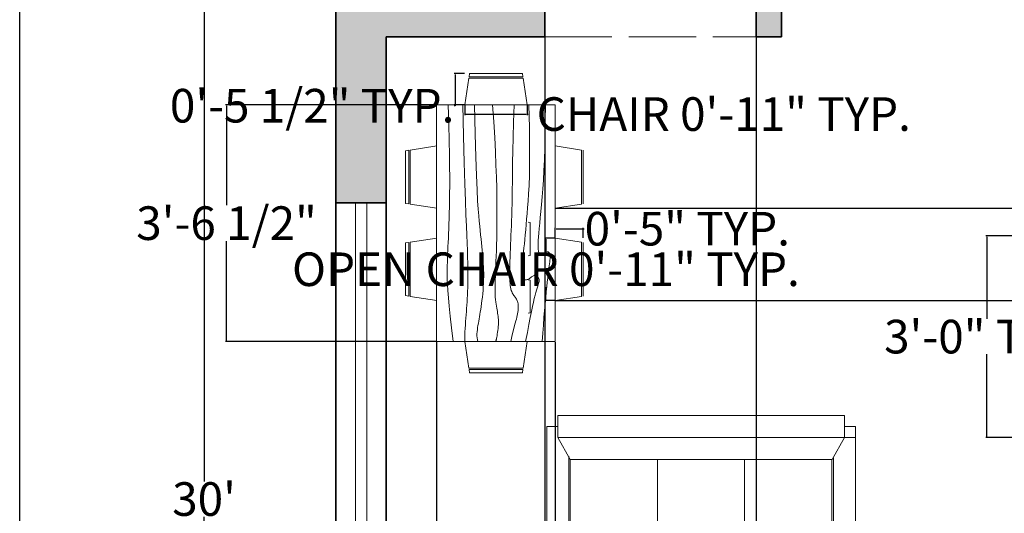
# Model space of a CAD drawing. Units: inches. Extents: x 335 to 688, y 1043 to 1486.
# Tile 3 of 7: x 335 to 510, y 1258 to 1347. Entities that reach past the tile are written whole.
import ezdxf

# ---------------------------------------------------------------- set-up
doc = ezdxf.new("R2010")
doc.units = ezdxf.units.IN
doc.header["$MEASUREMENT"] = 0
doc.linetypes.add('ACAD_ISO02W100', pattern=[15, 12, -3])
for name, color, linetype, lineweight in [('A-ANNO-DIMS', 2, 'Continuous', 18), ('A-ANNO-TTLB', 7, 'Continuous', 25), ('A-FURN', 8, 'Continuous', 18), ('A-GLAZ', 4, 'Continuous', 18), ('A-WALL', 7, 'Continuous', 35), ('A-WALL-OVHD', 7, 'ACAD_ISO02W100', 18), ('A-WALL-PATT', 252, 'Continuous', 13)]:
    doc.layers.add(name, color=color, linetype=linetype, lineweight=lineweight)
doc.styles.get("Standard").update_dxf_attribs({"font": 'arial.ttf'})
doc.dimstyles.get("Standard").update_dxf_attribs({"dimtxt": 6, "dimasz": 0.18, "dimexe": 0.18, "dimexo": 0.0625, "dimgap": 0.09, "dimtad": 0, "dimtih": 1, "dimtoh": 1, "dimdec": 1, "dimzin": 0, "dimdsep": 46, "dimlunit": 3, "dimtxsty": 'Standard', "dimcen": 0.09, "dimadec": 0, "dimazin": 0, "dimtfac": 1, "dimtdec": 1, "dimtofl": 0, "dimtmove": 0, "dimatfit": 3, "dimfxl": 1, "dimtolj": 1, "dimtzin": 0, "dimarcsym": 0})

# ---------------------------------------------------------------- blocks, each defined once
blk = doc.blocks.new('*D4')
at = {"layer": 'A-ANNO-DIMS', "color": 0, "lineweight": -2, "transparency": 16777216}
for p, q in [((391.04, 1440.97), (367.42, 1440.97)), ((367.6, 1440.79), (367.6, 1264.12)), ((367.6, 1081.15), (367.6, 1257.81)), ((391.04, 1080.97), (367.42, 1080.97))]:
    blk.add_line(p, q, dxfattribs=at)
at = {"layer": 'A-ANNO-DIMS', "color": 0, "transparency": 16777216}
for points in [[(367.57, 1440.79), (367.63, 1440.79), (367.6, 1440.97)], [(367.57, 1081.15), (367.63, 1081.15), (367.6, 1080.97)]]:
    blk.add_solid(points, dxfattribs=at)
at = {"layer": 'Defpoints', "color": 0, "transparency": 16777216}
for p in [(391.11, 1440.97), (367.6, 1080.97), (391.11, 1080.97)]:
    blk.add_point(p, dxfattribs=at)
at = {"layer": 'A-ANNO-DIMS', "color": 0, "transparency": 16777216, "insert": (367.6, 1260.97), "char_height": 6, "attachment_point": 5}
blk.add_mtext("\\A1;30'", dxfattribs=at)
blk = doc.blocks.new('SOFA-THREE-SEAT')
for p, q in [((53.08, 22.23), (1.96, 22.23)), ((1.96, 18.31), (1.96, 22.23)), ((53.08, 18.31), (53.08, 22.23)), ((0, 20.27), (0, 0)), ((1.96, 20.27), (0, 20.27)), ((55.04, 20.27), (53.08, 20.27)), ((55.04, 20.27), (55.04, 0)), ((55.04, 18.31), (1.96, 18.31)), ((4.17, 14.38), (1.96, 18.31)), ((53.08, 18.31), (50.88, 14.38)), ((3.92, 14.94), (3.92, 0)), ((19.74, 0.65), (19.74, 14.38)), ((35.3, 0.65), (35.3, 14.38)), ((50.87, 0.65), (50.87, 14.38)), ((51.12, 14.69), (51.12, 0)), ((3.92, 0), (0, 0)), ((51.12, 0), (55.04, 0))]:
    blk.add_line(p, q)
blk.add_lwpolyline([(50.88, 14.38), (4.17, 14.38), (4.17, 0.65), (50.87, 0.65)])
blk = doc.blocks.new('CHAIR-DINING')
for p, q in [((0.88, 10.41), (5.59, 11.15)), ((0, 10.28), (0.59, 10.37)), ((0, 10.28), (0, 0.87)), ((0.59, 0.78), (0.59, 10.37)), ((0.88, 10.41), (0.88, 0.73)), ((0.59, 0.78), (0, 0.87)), ((5.59, 0), (0.88, 0.73))]:
    blk.add_line(p, q)
blk = doc.blocks.new('CHAIR-DINING-OPEN')
for p, q in [((4.7, 10.41), (0, 11.15)), ((4.7, 10.41), (4.7, 0.73)), ((5, 0.78), (5, 10.37)), ((0, 0), (4.7, 0.73))]:
    blk.add_line(p, q)
blk = doc.blocks.new('WIN-60IN')
for p, q in [((0, 0), (0, 60)), ((3.5, 0), (3.5, 60)), ((5.5, 60), (5.5, 0)), ((9, 60), (9, 0))]:
    blk.add_line(p, q)
blk = doc.blocks.new('*D21')
at = {"layer": 'A-ANNO-DIMS', "color": 0, "lineweight": -2, "transparency": 16777216}
for p, q in [((414.1, 1331.32), (414.1, 1329.53)), ((425.25, 1331.32), (425.25, 1329.53)), ((414.28, 1329.71), (425.07, 1329.71)), ((425.25, 1329.71), (425.43, 1329.71))]:
    blk.add_line(p, q, dxfattribs=at)
at = {"layer": 'A-ANNO-DIMS', "color": 0, "transparency": 16777216}
for points in [[(414.28, 1329.74), (414.28, 1329.68), (414.1, 1329.71)], [(425.07, 1329.74), (425.07, 1329.68), (425.25, 1329.71)]]:
    blk.add_solid(points, dxfattribs=at)
at = {"layer": 'Defpoints', "color": 0, "transparency": 16777216}
for p in [(414.1, 1331.38), (425.25, 1331.38), (425.25, 1329.71)]:
    blk.add_point(p, dxfattribs=at)
at = {"layer": 'A-ANNO-DIMS', "color": 0, "transparency": 16777216, "insert": (460.3, 1329.71), "char_height": 6, "attachment_point": 5}
blk.add_mtext('\\A1;CHAIR 0\'-11" TYP.', dxfattribs=at)
blk = doc.blocks.new('*D22')
at = {"layer": 'A-ANNO-DIMS', "color": 0, "lineweight": -2, "transparency": 16777216}
for p, q in [((414.03, 1336.97), (412.24, 1336.97)), ((412.42, 1336.79), (412.42, 1331.56)), ((414.03, 1331.38), (412.24, 1331.38)), ((412.42, 1331.38), (412.42, 1331.2)), ((412.42, 1331.2), (412.24, 1331.2))]:
    blk.add_line(p, q, dxfattribs=at)
at = {"layer": 'A-ANNO-DIMS', "color": 0, "transparency": 16777216}
for points in [[(412.39, 1336.79), (412.45, 1336.79), (412.42, 1336.97)], [(412.39, 1331.56), (412.45, 1331.56), (412.42, 1331.38)]]:
    blk.add_solid(points, dxfattribs=at)
at = {"layer": 'Defpoints', "color": 0, "transparency": 16777216}
for p in [(414.1, 1336.97), (412.42, 1331.38), (414.1, 1331.38)]:
    blk.add_point(p, dxfattribs=at)
at = {"layer": 'A-ANNO-DIMS', "color": 0, "transparency": 16777216, "insert": (386.88, 1331.2), "char_height": 6, "attachment_point": 5}
blk.add_mtext('\\A1;0\'-5 1/2" TYP.', dxfattribs=at)
blk = doc.blocks.new('*D23')
at = {"layer": 'A-ANNO-DIMS', "color": 0, "lineweight": -2, "transparency": 16777216}
for p, q in [((430.19, 1307.57), (428.4, 1307.57)), ((428.58, 1307.39), (428.58, 1305.19)), ((428.58, 1296.6), (428.58, 1298.8)), ((430.19, 1296.42), (428.4, 1296.42))]:
    blk.add_line(p, q, dxfattribs=at)
at = {"layer": 'A-ANNO-DIMS', "color": 0, "transparency": 16777216}
for points in [[(428.55, 1307.39), (428.61, 1307.39), (428.58, 1307.57)], [(428.55, 1296.6), (428.61, 1296.6), (428.58, 1296.42)]]:
    blk.add_solid(points, dxfattribs=at)
at = {"layer": 'Defpoints', "color": 0, "transparency": 16777216}
for p in [(428.58, 1307.57), (430.25, 1307.57), (430.25, 1296.42)]:
    blk.add_point(p, dxfattribs=at)
at = {"layer": 'A-ANNO-DIMS', "color": 0, "transparency": 16777216, "insert": (428.58, 1302), "char_height": 6, "attachment_point": 5}
blk.add_mtext('\\A1;OPEN CHAIR 0\'-11" TYP.', dxfattribs=at)
blk = doc.blocks.new('*D24')
at = {"layer": 'A-ANNO-DIMS', "color": 0, "lineweight": -2, "transparency": 16777216}
for p, q in [((430.25, 1307.63), (430.25, 1309.42)), ((430.43, 1309.24), (435.07, 1309.24)), ((435.25, 1307.63), (435.25, 1309.42)), ((435.25, 1309.24), (435.43, 1309.24))]:
    blk.add_line(p, q, dxfattribs=at)
at = {"layer": 'A-ANNO-DIMS', "color": 0, "transparency": 16777216}
for points in [[(430.43, 1309.27), (430.43, 1309.21), (430.25, 1309.24)], [(435.07, 1309.27), (435.07, 1309.21), (435.25, 1309.24)]]:
    blk.add_solid(points, dxfattribs=at)
at = {"layer": 'Defpoints', "color": 0, "transparency": 16777216}
for p in [(435.25, 1309.24), (430.25, 1307.57), (435.25, 1307.57)]:
    blk.add_point(p, dxfattribs=at)
at = {"layer": 'A-ANNO-DIMS', "color": 0, "transparency": 16777216, "insert": (453.8, 1309.24), "char_height": 6, "attachment_point": 5}
blk.add_mtext('\\A1;0\'-5" TYP.', dxfattribs=at)
blk = doc.blocks.new('*D32')
at = {"layer": 'A-ANNO-DIMS', "color": 0, "lineweight": -2, "transparency": 16777216}
for p, q in [((512.54, 1307.97), (507.03, 1307.97)), ((507.21, 1307.79), (507.21, 1293.12)), ((507.21, 1272.15), (507.21, 1286.81)), ((512.54, 1271.97), (507.03, 1271.97))]:
    blk.add_line(p, q, dxfattribs=at)
at = {"layer": 'A-ANNO-DIMS', "color": 0, "transparency": 16777216}
for points in [[(507.18, 1307.79), (507.24, 1307.79), (507.21, 1307.97)], [(507.18, 1272.15), (507.24, 1272.15), (507.21, 1271.97)]]:
    blk.add_solid(points, dxfattribs=at)
at = {"layer": 'Defpoints', "color": 0, "transparency": 16777216}
for p in [(507.21, 1307.97), (512.61, 1307.97), (512.61, 1271.97)]:
    blk.add_point(p, dxfattribs=at)
at = {"layer": 'A-ANNO-DIMS', "color": 0, "transparency": 16777216, "insert": (507.21, 1289.97), "char_height": 6, "attachment_point": 5}
blk.add_mtext('\\A1;3\'-0" TYP.', dxfattribs=at)
blk = doc.blocks.new('*D39')
at = {"layer": 'A-ANNO-DIMS', "color": 0, "lineweight": -2, "transparency": 16777216}
for p, q in [((409.09, 1289), (409.09, 1061.29)), ((430.25, 1289), (430.25, 1061.29)), ((409.27, 1061.47), (411.89, 1061.47)), ((430.07, 1061.47), (427.45, 1061.47))]:
    blk.add_line(p, q, dxfattribs=at)
at = {"layer": 'A-ANNO-DIMS', "color": 0, "transparency": 16777216}
for points in [[(409.27, 1061.5), (409.27, 1061.44), (409.09, 1061.47)], [(430.07, 1061.5), (430.07, 1061.44), (430.25, 1061.47)]]:
    blk.add_solid(points, dxfattribs=at)
at = {"layer": 'Defpoints', "color": 0, "transparency": 16777216}
for p in [(409.09, 1289.07), (430.25, 1289.07), (430.25, 1061.47)]:
    blk.add_point(p, dxfattribs=at)
at = {"layer": 'A-ANNO-DIMS', "color": 0, "transparency": 16777216, "insert": (419.67, 1061.47), "char_height": 6, "attachment_point": 5}
blk.add_mtext('\\A1;1\'-9"', dxfattribs=at)
blk = doc.blocks.new('*D40')
at = {"layer": 'A-ANNO-DIMS', "color": 0, "lineweight": -2, "transparency": 16777216}
for p, q in [((409.03, 1331.38), (371.43, 1331.38)), ((371.61, 1331.2), (371.61, 1313.42)), ((371.61, 1289.25), (371.61, 1307.03)), ((409.03, 1289.07), (371.43, 1289.07))]:
    blk.add_line(p, q, dxfattribs=at)
at = {"layer": 'A-ANNO-DIMS', "color": 0, "transparency": 16777216}
for points in [[(371.58, 1331.2), (371.64, 1331.2), (371.61, 1331.38)], [(371.58, 1289.25), (371.64, 1289.25), (371.61, 1289.07)]]:
    blk.add_solid(points, dxfattribs=at)
at = {"layer": 'Defpoints', "color": 0, "transparency": 16777216}
for p in [(371.61, 1331.38), (409.09, 1331.38), (409.09, 1289.07)]:
    blk.add_point(p, dxfattribs=at)
at = {"layer": 'A-ANNO-DIMS', "color": 0, "transparency": 16777216, "insert": (371.61, 1310.23), "char_height": 6, "attachment_point": 5}
blk.add_mtext('\\A1;3\'-6 1/2"', dxfattribs=at)
blk = doc.blocks.new('*D41')
at = {"layer": 'A-ANNO-DIMS', "color": 0, "lineweight": -2, "transparency": 16777216}
for p, q in [((430.31, 1312.88), (650.79, 1312.88)), ((650.61, 1312.7), (650.61, 1307.84)), ((650.61, 1296.6), (650.61, 1301.46)), ((430.31, 1296.42), (650.79, 1296.42))]:
    blk.add_line(p, q, dxfattribs=at)
at = {"layer": 'A-ANNO-DIMS', "color": 0, "transparency": 16777216}
for points in [[(650.58, 1312.7), (650.64, 1312.7), (650.61, 1312.88)], [(650.58, 1296.6), (650.64, 1296.6), (650.61, 1296.42)]]:
    blk.add_solid(points, dxfattribs=at)
at = {"layer": 'Defpoints', "color": 0, "transparency": 16777216}
for p in [(430.25, 1312.88), (650.61, 1312.88), (430.25, 1296.42)]:
    blk.add_point(p, dxfattribs=at)
at = {"layer": 'A-ANNO-DIMS', "color": 0, "transparency": 16777216, "insert": (650.61, 1304.65), "char_height": 6, "attachment_point": 5}
blk.add_mtext('\\A1;1\'-4 1/2"', dxfattribs=at)
blk = doc.blocks.new('*D60')
at = {"layer": 'A-ANNO-DIMS', "color": 0, "lineweight": -2, "transparency": 16777216}
for p, q in [((400.11, 1343.4), (400.11, 1061.29)), ((428.36, 1343.4), (428.36, 1061.29)), ((400.29, 1061.47), (428.18, 1061.47)), ((428.36, 1061.47), (428.54, 1061.47))]:
    blk.add_line(p, q, dxfattribs=at)
at = {"layer": 'A-ANNO-DIMS', "color": 0, "transparency": 16777216}
for points in [[(400.29, 1061.5), (400.29, 1061.44), (400.11, 1061.47)], [(428.18, 1061.5), (428.18, 1061.44), (428.36, 1061.47)]]:
    blk.add_solid(points, dxfattribs=at)
at = {"layer": 'Defpoints', "color": 0, "transparency": 16777216}
for p in [(400.11, 1343.47), (428.36, 1343.47), (428.36, 1061.47)]:
    blk.add_point(p, dxfattribs=at)
at = {"layer": 'A-ANNO-DIMS', "color": 0, "transparency": 16777216, "insert": (443.65, 1061.47), "char_height": 6, "attachment_point": 5}
blk.add_mtext('\\A1;2\'-4 1/2"', dxfattribs=at)
blk = doc.blocks.new('*D61')
at = {"layer": 'A-ANNO-DIMS', "color": 0, "lineweight": -2, "transparency": 16777216}
for p, q in [((428.36, 1347.9), (428.36, 1061.29)), ((466.11, 1347.9), (466.11, 1061.29)), ((428.54, 1061.47), (432.18, 1061.47)), ((465.93, 1061.47), (462.29, 1061.47))]:
    blk.add_line(p, q, dxfattribs=at)
at = {"layer": 'A-ANNO-DIMS', "color": 0, "transparency": 16777216}
for points in [[(428.54, 1061.5), (428.54, 1061.44), (428.36, 1061.47)], [(465.93, 1061.5), (465.93, 1061.44), (466.11, 1061.47)]]:
    blk.add_solid(points, dxfattribs=at)
at = {"layer": 'Defpoints', "color": 0, "transparency": 16777216}
for p in [(428.36, 1347.97), (466.11, 1347.97), (466.11, 1061.47)]:
    blk.add_point(p, dxfattribs=at)
at = {"layer": 'A-ANNO-DIMS', "color": 0, "transparency": 16777216, "insert": (447.24, 1061.47), "char_height": 6, "attachment_point": 5}
blk.add_mtext('\\A1;3\'-1 1/2"', dxfattribs=at)

msp = doc.modelspace()

# ---------------------------------------------------------------- hatches: boundary and pattern name
at = {"layer": 'A-WALL-PATT'}
h = msp.add_hatch(color=256, dxfattribs=at)
h.dxf.hatch_style = 1
h.paths.add_polyline_path([(478.71, 1440.97), (391.11, 1440.97), (391.11, 1411.42), (400.11, 1411.42), (400.11, 1431.97), (466.11, 1431.97), (466.11, 1347.97), (466.11, 1343.47), (470.61, 1343.47), (470.61, 1367.47), (512.61, 1367.47), (512.61, 1350.97), (517.11, 1350.97), (517.11, 1372.97), (512.61, 1372.97), (512.61, 1371.97), (470.61, 1371.97), (470.61, 1431.97), (478.71, 1431.97)])
h.paths.add_polyline_path([(631.11, 1440.97), (502.71, 1440.97), (502.71, 1431.97), (512.61, 1431.97), (512.61, 1404.97), (517.11, 1404.97), (517.11, 1431.97), (622.11, 1431.97), (622.11, 1401.6), (631.11, 1401.6)])
h.paths.add_polyline_path([(631.11, 1341.6), (622.11, 1341.6), (622.11, 1313.47), (517.11, 1313.47), (517.11, 1314.47), (512.61, 1314.47), (512.61, 1313.47), (512.61, 1307.97), (517.11, 1307.97), (517.11, 1308.97), (553.11, 1308.97), (553.11, 1262.47), (558.61, 1262.47), (558.61, 1266.97), (557.61, 1266.97), (557.61, 1308.97), (622.11, 1308.97), (622.11, 1297.63), (631.11, 1297.63)])
h.paths.add_polyline_path([(631.11, 1273.63), (622.11, 1273.63), (622.11, 1266.97), (590.61, 1266.97), (590.61, 1262.47), (622.11, 1262.47), (622.11, 1230.86), (631.11, 1230.86)])
h.paths.add_polyline_path([(400.11, 1253.85), (391.11, 1253.85), (391.11, 1132.26), (400.11, 1132.26), (400.11, 1149.97), (411.11, 1149.97), (411.11, 1154.47), (400.11, 1154.47)], flags=17)
h.paths.add_polyline_path([(400.11, 1375.42), (391.11, 1375.42), (391.11, 1313.85), (400.11, 1313.85), (400.11, 1343.47), (428.36, 1343.47), (428.36, 1347.97), (400.11, 1347.97)])

# ---------------------------------------------------------------- linework, layer by layer
at = {"layer": 'A-ANNO-TTLB'}
msp.add_lwpolyline([(334.72, 1486.4), (681.01, 1486.4), (681.01, 1043.03), (334.72, 1043.03)], close=True, dxfattribs=at)
at = {"layer": 'A-FURN'}
for p, q in [((409.09, 1331.38), (409.09, 1289.07)), ((430.25, 1331.38), (409.09, 1331.38)), ((430.25, 1289.07), (430.25, 1331.38)), ((425.76, 1310.32), (425.4, 1310.38)), ((425.76, 1310.32), (425.76, 1304.46)), ((425.4, 1304.4), (425.76, 1304.46)), ((425.76, 1300.06), (425.4, 1300.12)), ((425.76, 1300.06), (425.76, 1294.2)), ((425.4, 1294.14), (425.76, 1294.2)), ((409.09, 1289.07), (430.25, 1289.07))]:
    msp.add_line(p, q, dxfattribs=at)
for points in [[(411.15, 1331.38), (411.25, 1327.91), (411.32, 1324.94), (411.37, 1322.41), (411.4, 1320.26), (411.42, 1318.44), (411.42, 1316.87), (411.41, 1315.5), (411.39, 1314.27), (411.37, 1313.12), (411.35, 1312.04), (411.32, 1311.03), (411.29, 1310.08), (411.26, 1309.19), (411.22, 1308.35), (411.19, 1307.55), (411.15, 1306.8), (411.11, 1306.08), (411.08, 1305.39), (411.05, 1304.71), (411.02, 1304.03), (411, 1303.34), (410.98, 1302.63), (410.97, 1301.88), (410.98, 1301.09), (410.99, 1300.24), (411.03, 1299.29), (411.09, 1298.19), (411.18, 1296.91), (411.32, 1295.4), (411.5, 1293.61), (411.73, 1291.52), (412.03, 1289.07)], [(413.79, 1331.38), (413.9, 1325.74), (414.01, 1321.08), (414.12, 1317.27), (414.22, 1314.19), (414.31, 1311.71), (414.39, 1309.71), (414.47, 1308.06), (414.53, 1306.65), (414.58, 1305.36), (414.61, 1304.17), (414.64, 1303.07), (414.65, 1302.06), (414.66, 1301.12), (414.65, 1300.26), (414.64, 1299.46), (414.63, 1298.72), (414.61, 1298.02), (414.58, 1297.37), (414.55, 1296.76), (414.52, 1296.16), (414.48, 1295.59), (414.44, 1295.02), (414.4, 1294.45), (414.36, 1293.87), (414.31, 1293.27), (414.26, 1292.66), (414.22, 1292.05), (414.18, 1291.43), (414.14, 1290.82), (414.11, 1290.22), (414.09, 1289.63), (414.09, 1289.07)], [(415.85, 1331.38), (415.96, 1326.2), (416.07, 1322.03), (416.18, 1318.73), (416.29, 1316.17), (416.39, 1314.21), (416.49, 1312.72), (416.59, 1311.56), (416.68, 1310.59), (416.77, 1309.71), (416.86, 1308.89), (416.94, 1308.12), (417.01, 1307.39), (417.09, 1306.7), (417.15, 1306.04), (417.21, 1305.4), (417.27, 1304.79), (417.32, 1304.19), (417.37, 1303.6), (417.41, 1303.02), (417.44, 1302.44), (417.47, 1301.86), (417.48, 1301.28), (417.48, 1300.69), (417.47, 1300.09), (417.44, 1299.48), (417.41, 1298.86), (417.36, 1298.24), (417.3, 1297.62), (417.24, 1297.02), (417.17, 1296.43), (417.1, 1295.87), (417.03, 1295.34), (416.95, 1294.84), (416.88, 1294.37), (416.81, 1293.94), (416.74, 1293.52), (416.66, 1293.12), (416.6, 1292.74), (416.53, 1292.36), (416.46, 1291.98), (416.4, 1291.6), (416.35, 1291.23), (416.3, 1290.85), (416.28, 1290.48), (416.27, 1290.11), (416.29, 1289.75), (416.35, 1289.4), (416.44, 1289.07)], [(419.08, 1331.38), (419.28, 1328.32), (419.45, 1325.52), (419.58, 1322.95), (419.67, 1320.6), (419.75, 1318.45), (419.8, 1316.49), (419.83, 1314.68), (419.84, 1313.02), (419.85, 1311.48), (419.84, 1310.06), (419.82, 1308.74), (419.8, 1307.51), (419.77, 1306.37), (419.74, 1305.31), (419.71, 1304.31), (419.67, 1303.37), (419.63, 1302.47), (419.6, 1301.62), (419.57, 1300.82), (419.54, 1300.07), (419.52, 1299.36), (419.51, 1298.71), (419.51, 1298.1), (419.52, 1297.54), (419.55, 1297.03), (419.59, 1296.57), (419.63, 1296.15), (419.68, 1295.76), (419.74, 1295.4), (419.8, 1295.07), (419.86, 1294.75), (419.92, 1294.45), (419.97, 1294.17), (420.02, 1293.88), (420.06, 1293.6), (420.09, 1293.32), (420.11, 1293.03), (420.12, 1292.73), (420.12, 1292.43), (420.11, 1292.1), (420.09, 1291.77), (420.05, 1291.42), (420.01, 1291.07), (419.96, 1290.74), (419.91, 1290.42), (419.86, 1290.13), (419.81, 1289.88), (419.77, 1289.68), (419.74, 1289.53), (419.71, 1289.43), (419.7, 1289.36), (419.68, 1289.31), (419.68, 1289.27), (419.67, 1289.22), (419.67, 1289.16), (419.67, 1289.07)], [(422.9, 1331.38), (422.81, 1328.28), (422.73, 1325.55), (422.68, 1323.15), (422.64, 1321.06), (422.61, 1319.22), (422.59, 1317.6), (422.58, 1316.17), (422.56, 1314.88), (422.54, 1313.7), (422.52, 1312.61), (422.49, 1311.6), (422.46, 1310.66), (422.42, 1309.77), (422.39, 1308.92), (422.35, 1308.1), (422.32, 1307.29), (422.28, 1306.48), (422.24, 1305.68), (422.21, 1304.89), (422.18, 1304.13), (422.16, 1303.39), (422.14, 1302.69), (422.12, 1302.02), (422.12, 1301.41), (422.12, 1300.85), (422.14, 1300.34), (422.16, 1299.88), (422.19, 1299.47), (422.23, 1299.1), (422.29, 1298.77), (422.35, 1298.48), (422.41, 1298.23), (422.49, 1298), (422.58, 1297.81), (422.67, 1297.63), (422.76, 1297.48), (422.86, 1297.34), (422.96, 1297.21), (423.05, 1297.08), (423.15, 1296.95), (423.24, 1296.82), (423.32, 1296.68), (423.4, 1296.54), (423.47, 1296.38), (423.53, 1296.22), (423.58, 1296.04), (423.61, 1295.84), (423.64, 1295.63), (423.65, 1295.4), (423.65, 1295.16), (423.63, 1294.89), (423.61, 1294.62), (423.57, 1294.33), (423.52, 1294.04), (423.46, 1293.74), (423.39, 1293.43), (423.32, 1293.11), (423.23, 1292.77), (423.12, 1292.38), (423, 1291.93), (422.86, 1291.39), (422.7, 1290.75), (422.52, 1289.98), (422.32, 1289.07)], [(425.55, 1331.38), (425.63, 1327.26), (425.67, 1323.85), (425.66, 1321.05), (425.63, 1318.79), (425.57, 1316.95), (425.49, 1315.44), (425.4, 1314.17), (425.3, 1313.04), (425.21, 1311.97), (425.13, 1310.95), (425.05, 1309.97), (424.97, 1309.04), (424.89, 1308.15), (424.81, 1307.32), (424.74, 1306.54), (424.67, 1305.82), (424.59, 1305.15), (424.52, 1304.53), (424.45, 1303.96), (424.39, 1303.45), (424.34, 1302.98), (424.29, 1302.56), (424.25, 1302.18), (424.23, 1301.85), (424.21, 1301.56), (424.22, 1301.3), (424.23, 1301.08), (424.26, 1300.9), (424.29, 1300.73), (424.34, 1300.6), (424.4, 1300.48), (424.47, 1300.38), (424.55, 1300.3), (424.63, 1300.23), (424.73, 1300.17), (424.83, 1300.13), (424.93, 1300.11), (425.04, 1300.1), (425.14, 1300.11), (425.25, 1300.14), (425.36, 1300.18), (425.48, 1300.24), (425.59, 1300.31), (425.7, 1300.39), (425.81, 1300.48), (425.92, 1300.56), (426.03, 1300.65), (426.14, 1300.72), (426.25, 1300.79), (426.36, 1300.85), (426.46, 1300.9), (426.57, 1300.93), (426.68, 1300.94), (426.78, 1300.94), (426.87, 1300.91), (426.97, 1300.87), (427.06, 1300.8), (427.14, 1300.72), (427.21, 1300.61), (427.28, 1300.49), (427.32, 1300.34), (427.35, 1300.19), (427.37, 1300.02), (427.36, 1299.84), (427.33, 1299.65), (427.28, 1299.45), (427.21, 1299.21), (427.13, 1298.95), (427.02, 1298.64), (426.91, 1298.28), (426.78, 1297.86), (426.65, 1297.37), (426.51, 1296.8), (426.36, 1296.14), (426.19, 1295.37), (426, 1294.46), (425.79, 1293.39), (425.55, 1292.15), (425.27, 1290.72), (424.96, 1289.07)], [(428.49, 1331.38), (428.47, 1328.55), (428.44, 1325.98), (428.38, 1323.66), (428.3, 1321.56), (428.21, 1319.65), (428.12, 1317.92), (428.01, 1316.35), (427.9, 1314.9), (427.79, 1313.57), (427.68, 1312.34), (427.58, 1311.22), (427.48, 1310.2), (427.4, 1309.29), (427.32, 1308.47), (427.26, 1307.76), (427.21, 1307.14), (427.19, 1306.62), (427.18, 1306.18), (427.18, 1305.82), (427.2, 1305.54), (427.24, 1305.31), (427.28, 1305.13), (427.34, 1304.99), (427.41, 1304.89), (427.49, 1304.81), (427.57, 1304.75), (427.66, 1304.71), (427.76, 1304.69), (427.86, 1304.68), (427.95, 1304.69), (428.05, 1304.71), (428.14, 1304.74), (428.23, 1304.78), (428.32, 1304.83), (428.4, 1304.88), (428.48, 1304.93), (428.56, 1304.98), (428.63, 1305.02), (428.71, 1305.06), (428.78, 1305.08), (428.85, 1305.09), (428.93, 1305.09), (429, 1305.08), (429.06, 1305.05), (429.12, 1305), (429.18, 1304.95), (429.23, 1304.87), (429.27, 1304.79), (429.3, 1304.69), (429.33, 1304.57), (429.34, 1304.44), (429.34, 1304.28), (429.34, 1304.09), (429.33, 1303.87), (429.3, 1303.61), (429.27, 1303.32), (429.23, 1302.99), (429.18, 1302.6), (429.12, 1302.17), (429.06, 1301.66), (428.98, 1301.09), (428.91, 1300.44), (428.82, 1299.71), (428.73, 1298.89), (428.64, 1297.97), (428.54, 1296.95), (428.44, 1295.84), (428.33, 1294.65), (428.23, 1293.37), (428.12, 1292.01), (428.01, 1290.57), (427.9, 1289.07)]]:
    msp.add_lwpolyline(points, dxfattribs=at)
at = {"layer": 'A-WALL'}
for p, q in [((391.11, 1440.97), (391.11, 1080.97)), ((470.61, 1367.47), (470.61, 1343.47)), ((428.36, 1347.97), (428.36, 1343.47)), ((466.11, 1347.97), (466.11, 1343.47)), ((400.11, 1343.47), (428.36, 1343.47)), ((400.11, 1343.47), (400.11, 1154.47)), ((466.11, 1343.47), (470.61, 1343.47)), ((391.11, 1313.85), (400.11, 1313.85))]:
    msp.add_line(p, q, dxfattribs=at)
at = {"layer": 'A-WALL-OVHD'}
msp.add_line((428.36, 1343.47), (466.11, 1343.47), dxfattribs=at)

# ---------------------------------------------------------------- block references
at = {"layer": 'A-FURN', "rotation": 270}
msp.add_blockref('CHAIR-DINING', (414.1, 1336.97), dxfattribs=at)
at = {"layer": 'A-FURN'}
for name, p in [('CHAIR-DINING', (403.51, 1312.88)), ('CHAIR-DINING-OPEN', (430.25, 1312.88)), ('CHAIR-DINING', (403.51, 1296.42)), ('CHAIR-DINING-OPEN', (430.25, 1296.42)), ('SOFA-THREE-SEAT', (428.73, 1253.66))]:
    msp.add_blockref(name, p, dxfattribs=at)
at = {"layer": 'A-FURN', "extrusion": (0, 0, -1), "zscale": -1, "rotation": 90}
msp.add_blockref('CHAIR-DINING', (-414.1, 1283.48), dxfattribs=at)
at = {"layer": 'A-GLAZ'}
msp.add_blockref('WIN-60IN', (391.11, 1253.85), dxfattribs=at)

# ---------------------------------------------------------------- dimensions: what is measured, and where the dimension line sits
at = {"layer": 'A-ANNO-DIMS'}
for base, p1, p2, override, picture, middle in [((367.6, 1080.97), (391.11, 1440.97), (391.11, 1080.97), {"dimclrd": 0, "dimclre": 0, "dimclrt": 0}, '*D4', (367.6, 1260.97)), ((371.61, 1331.38), (409.09, 1289.07), (409.09, 1331.38), {"dimdec": 1, "dimlfac": 1, "dimrnd": 0, "dimzin": 1, "dimdsep": 46, "dimlunit": 4, "dimfrac": 2}, '*D40', (371.61, 1310.23)), ((650.61, 1312.88), (430.25, 1296.42), (430.25, 1312.88), {"dimdec": 1, "dimlfac": 1, "dimrnd": 0, "dimzin": 1, "dimdsep": 46, "dimlunit": 4, "dimfrac": 2}, '*D41', (650.61, 1304.65))]:
    dim = msp.add_linear_dim(base=base, p1=p1, p2=p2, angle=90, dimstyle='Standard', override=override, dxfattribs=at)
    dim.commit()
    dim.dimension.update_dxf_attribs({"geometry": picture, "text_midpoint": middle})
for base, p1, p2, picture, middle in [((466.1064, 1061.4667), (428.3646, 1347.9667), (466.1064, 1347.9667), '*D61', (447.2355, 1061.4667)), ((428.3646, 1061.4667), (400.1064, 1343.4667), (428.3646, 1343.4667), '*D60', (443.651, 1061.4667)), ((430.25, 1061.47), (409.09, 1289.07), (430.25, 1289.07), '*D39', (419.67, 1061.47))]:
    dim = msp.add_linear_dim(base=base, p1=p1, p2=p2, dimstyle='Standard', override={"dimdec": 1, "dimlfac": 1, "dimrnd": 0, "dimzin": 1, "dimdsep": 46, "dimlunit": 4, "dimfrac": 2}, dxfattribs=at)
    dim.commit()
    dim.dimension.update_dxf_attribs({"geometry": picture, "text_midpoint": middle})
for base, p1, p2, angle, text, picture, middle in [((412.42, 1331.38), (414.1, 1336.97), (414.1, 1331.38), 270, '<> TYP.', '*D22', (386.88, 1331.2)), ((428.5767, 1307.5721), (430.2491, 1296.4229), (430.2491, 1307.5721), 90, 'OPEN CHAIR <> TYP.', '*D23', (428.5767, 1301.9975)), ((507.21, 1307.97), (512.61, 1271.97), (512.61, 1307.97), 90, '<> TYP.', '*D32', (507.21, 1289.97))]:
    dim = msp.add_linear_dim(base=base, p1=p1, p2=p2, angle=angle, text=text, dimstyle='Standard', override={"dimdec": 1, "dimlfac": 1, "dimrnd": 0, "dimzin": 1, "dimdsep": 46, "dimlunit": 4, "dimfrac": 2}, dxfattribs=at)
    dim.commit()
    dim.dimension.update_dxf_attribs({"geometry": picture, "text_midpoint": middle})
for base, p1, p2, text, picture, middle in [((425.2457, 1329.7109), (414.0965, 1331.3833), (425.2457, 1331.3833), 'CHAIR <> TYP.', '*D21', (460.3022, 1329.7109)), ((435.25, 1309.24), (430.25, 1307.57), (435.25, 1307.57), '<> TYP.', '*D24', (453.8, 1309.24))]:
    dim = msp.add_linear_dim(base=base, p1=p1, p2=p2, text=text, dimstyle='Standard', override={"dimdec": 1, "dimlfac": 1, "dimrnd": 0, "dimzin": 1, "dimdsep": 46, "dimlunit": 4, "dimfrac": 2}, dxfattribs=at)
    dim.commit()
    dim.dimension.update_dxf_attribs({"geometry": picture, "text_midpoint": middle})

doc.saveas('drawing.dxf')
